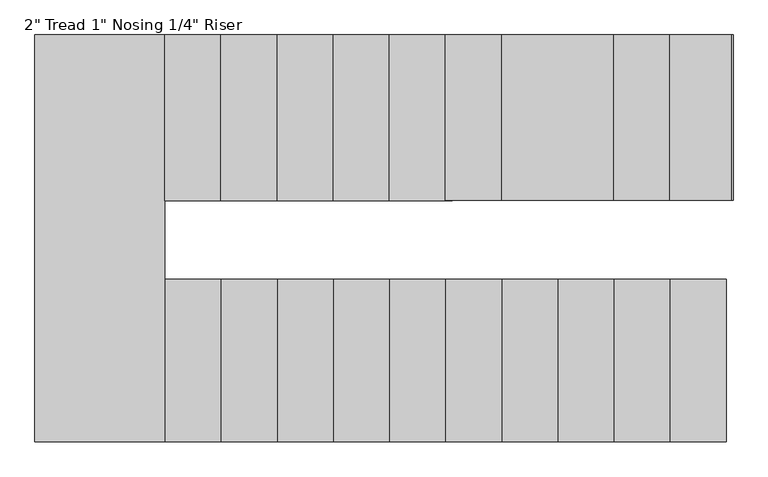
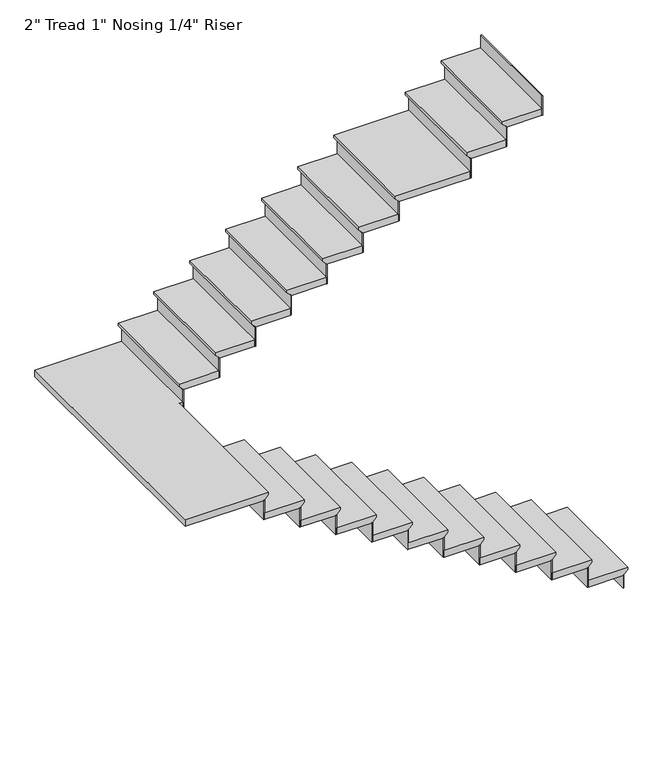
"""IFC4 building model written with IfcOpenShell, lengths in millimetres: stair flight geometry."""

from ifc_helpers import new_model, si_unit, origin, place, context, project, spatial, faceted_brep, source, transform, mapped, element, save


def stair_flight_03342cd4(model_context):
    return source(origin(), model_context, "Body", "Brep", [
        faceted_brep([(-3117.2664982, -7431.6600272, 9270.0928571), (-3117.2664982, -7431.6600272, 9289.1428571), (-3117.2664982, -8168.2600272, 9289.1428571), (-3117.2664982, -8168.2600272, 9270.0928571), (-3142.6664982, -7431.6600272, 9244.6928571), (-3142.6664982, -8168.2600272, 9244.6928571), (-3396.6664982, -7431.6600272, 9289.1428571), (-3396.6664982, -8168.2600272, 9289.1428571), (-3142.6664982, -8168.2600272, 9238.3428571), (-3396.6664982, -8168.2600272, 9238.3428571), (-3396.6664982, -7431.6600272, 9238.3428571), (-3142.6664982, -7431.6600272, 9238.3428571)], [[[0, 1, 2, 3]], [[4, 0, 3, 5]], [[2, 1, 6, 7]], [[8, 9, 10, 11]], [[2, 7, 9, 8, 5, 3]], [[8, 11, 4, 5]], [[6, 1, 0, 4, 11, 10]], [[7, 6, 10, 9]]]),
        faceted_brep([(-3142.6664982, -7431.6600272, 9238.3428571), (-3142.6664982, -7431.6600272, 9144.0), (-3149.0164982, -7431.6600272, 9144.0), (-3149.0164982, -7431.6600272, 9238.3428571), (-3142.6664982, -8168.2600272, 9238.3428571), (-3149.0164982, -8168.2600272, 9238.3428571), (-3149.0164982, -8168.2600272, 9144.0), (-3142.6664982, -8168.2600272, 9144.0)], [[[0, 1, 2, 3]], [[4, 5, 6, 7]], [[1, 0, 4, 7]], [[2, 1, 7, 6]], [[3, 2, 6, 5]], [[0, 3, 5, 4]]]),
        faceted_brep([(-3396.6664982, -7431.6600272, 9383.4857143), (-3396.6664982, -7431.6600272, 9238.3428571), (-3403.0164982, -7431.6600272, 9238.3428571), (-3403.0164982, -7431.6600272, 9383.4857143), (-3396.6664982, -8168.2600272, 9383.4857143), (-3403.0164982, -8168.2600272, 9383.4857143), (-3403.0164982, -8168.2600272, 9238.3428571), (-3396.6664982, -8168.2600272, 9238.3428571)], [[[0, 1, 2, 3]], [[4, 5, 6, 7]], [[1, 0, 4, 7]], [[2, 1, 7, 6]], [[3, 2, 6, 5]], [[0, 3, 5, 4]]]),
        faceted_brep([(-3371.2664982, -8168.2600272, 9434.2857143), (-3371.2664982, -7431.6600272, 9434.2857143), (-3650.6664982, -7431.6600272, 9434.2857143), (-3650.6664982, -8168.2600272, 9434.2857143), (-3396.6664982, -8168.2600272, 9383.4857143), (-3650.6664982, -8168.2600272, 9383.4857143), (-3650.6664982, -7431.6600272, 9383.4857143), (-3396.6664982, -7431.6600272, 9383.4857143), (-3396.6664982, -8168.2600272, 9389.8357143), (-3371.2664982, -8168.2600272, 9415.2357143), (-3396.6664982, -7431.6600272, 9389.8357143), (-3371.2664982, -7431.6600272, 9415.2357143)], [[[0, 1, 2, 3]], [[4, 5, 6, 7]], [[0, 3, 5, 4, 8, 9]], [[4, 7, 10, 8]], [[2, 1, 11, 10, 7, 6]], [[3, 2, 6, 5]], [[11, 1, 0, 9]], [[10, 11, 9, 8]]]),
        faceted_brep([(-3650.6664982, -7431.6600272, 9528.6285714), (-3650.6664982, -7431.6600272, 9383.4857143), (-3657.0164982, -7431.6600272, 9383.4857143), (-3657.0164982, -7431.6600272, 9528.6285714), (-3650.6664982, -8168.2600272, 9528.6285714), (-3657.0164982, -8168.2600272, 9528.6285714), (-3657.0164982, -8168.2600272, 9383.4857143), (-3650.6664982, -8168.2600272, 9383.4857143)], [[[0, 1, 2, 3]], [[4, 5, 6, 7]], [[1, 0, 4, 7]], [[2, 1, 7, 6]], [[3, 2, 6, 5]], [[0, 3, 5, 4]]]),
        faceted_brep([(-3625.2664982, -8168.2600272, 9579.4285714), (-3625.2664982, -7431.6600272, 9579.4285714), (-3904.6664982, -7431.6600272, 9579.4285714), (-3904.6664982, -8168.2600272, 9579.4285714), (-3650.6664982, -8168.2600272, 9528.6285714), (-3904.6664982, -8168.2600272, 9528.6285714), (-3904.6664982, -7431.6600272, 9528.6285714), (-3650.6664982, -7431.6600272, 9528.6285714), (-3650.6664982, -8168.2600272, 9534.9785714), (-3625.2664982, -8168.2600272, 9560.3785714), (-3650.6664982, -7431.6600272, 9534.9785714), (-3625.2664982, -7431.6600272, 9560.3785714)], [[[0, 1, 2, 3]], [[4, 5, 6, 7]], [[0, 3, 5, 4, 8, 9]], [[4, 7, 10, 8]], [[2, 1, 11, 10, 7, 6]], [[3, 2, 6, 5]], [[11, 1, 0, 9]], [[10, 11, 9, 8]]]),
        faceted_brep([(-3904.6664982, -7431.6600272, 9673.7714286), (-3904.6664982, -7431.6600272, 9528.6285714), (-3911.0164982, -7431.6600272, 9528.6285714), (-3911.0164982, -7431.6600272, 9673.7714286), (-3904.6664982, -8168.2600272, 9673.7714286), (-3911.0164982, -8168.2600272, 9673.7714286), (-3911.0164982, -8168.2600272, 9528.6285714), (-3904.6664982, -8168.2600272, 9528.6285714)], [[[0, 1, 2, 3]], [[4, 5, 6, 7]], [[1, 0, 4, 7]], [[2, 1, 7, 6]], [[3, 2, 6, 5]], [[0, 3, 5, 4]]]),
        faceted_brep([(-3879.2664982, -8168.2600272, 9724.5714286), (-3879.2664982, -7431.6600272, 9724.5714286), (-4158.6664982, -7431.6600272, 9724.5714286), (-4158.6664982, -8168.2600272, 9724.5714286), (-3904.6664982, -8168.2600272, 9673.7714286), (-4158.6664982, -8168.2600272, 9673.7714286), (-4158.6664982, -7431.6600272, 9673.7714286), (-3904.6664982, -7431.6600272, 9673.7714286), (-3904.6664982, -8168.2600272, 9680.1214286), (-3879.2664982, -8168.2600272, 9705.5214286), (-3904.6664982, -7431.6600272, 9680.1214286), (-3879.2664982, -7431.6600272, 9705.5214286)], [[[0, 1, 2, 3]], [[4, 5, 6, 7]], [[0, 3, 5, 4, 8, 9]], [[4, 7, 10, 8]], [[2, 1, 11, 10, 7, 6]], [[3, 2, 6, 5]], [[11, 1, 0, 9]], [[10, 11, 9, 8]]]),
        faceted_brep([(-4158.6664982, -7431.6600272, 9818.9142857), (-4158.6664982, -7431.6600272, 9673.7714286), (-4165.0164982, -7431.6600272, 9673.7714286), (-4165.0164982, -7431.6600272, 9818.9142857), (-4158.6664982, -8168.2600272, 9818.9142857), (-4165.0164982, -8168.2600272, 9818.9142857), (-4165.0164982, -8168.2600272, 9673.7714286), (-4158.6664982, -8168.2600272, 9673.7714286)], [[[0, 1, 2, 3]], [[4, 5, 6, 7]], [[1, 0, 4, 7]], [[2, 1, 7, 6]], [[3, 2, 6, 5]], [[0, 3, 5, 4]]]),
        faceted_brep([(-4133.2664982, -8168.2600272, 9869.7142857), (-4133.2664982, -7431.6600272, 9869.7142857), (-4412.6664982, -7431.6600272, 9869.7142857), (-4412.6664982, -8168.2600272, 9869.7142857), (-4158.6664982, -8168.2600272, 9818.9142857), (-4412.6664982, -8168.2600272, 9818.9142857), (-4412.6664982, -7431.6600272, 9818.9142857), (-4158.6664982, -7431.6600272, 9818.9142857), (-4158.6664982, -8168.2600272, 9825.2642857), (-4133.2664982, -8168.2600272, 9850.6642857), (-4158.6664982, -7431.6600272, 9825.2642857), (-4133.2664982, -7431.6600272, 9850.6642857)], [[[0, 1, 2, 3]], [[4, 5, 6, 7]], [[0, 3, 5, 4, 8, 9]], [[4, 7, 10, 8]], [[2, 1, 11, 10, 7, 6]], [[3, 2, 6, 5]], [[11, 1, 0, 9]], [[10, 11, 9, 8]]]),
        faceted_brep([(-4412.6664982, -7431.6600272, 9964.0571429), (-4412.6664982, -7431.6600272, 9818.9142857), (-4419.0164982, -7431.6600272, 9818.9142857), (-4419.0164982, -7431.6600272, 9964.0571429), (-4412.6664982, -8168.2600272, 9964.0571429), (-4419.0164982, -8168.2600272, 9964.0571429), (-4419.0164982, -8168.2600272, 9818.9142857), (-4412.6664982, -8168.2600272, 9818.9142857)], [[[0, 1, 2, 3]], [[4, 5, 6, 7]], [[1, 0, 4, 7]], [[2, 1, 7, 6]], [[3, 2, 6, 5]], [[0, 3, 5, 4]]]),
        faceted_brep([(-4387.2664982, -8168.2600272, 10014.8571429), (-4387.2664982, -7431.6600272, 10014.8571429), (-4666.6664982, -7431.6600272, 10014.8571429), (-4666.6664982, -8168.2600272, 10014.8571429), (-4412.6664982, -8168.2600272, 9964.0571429), (-4666.6664982, -8168.2600272, 9964.0571429), (-4666.6664982, -7431.6600272, 9964.0571429), (-4412.6664982, -7431.6600272, 9964.0571429), (-4412.6664982, -8168.2600272, 9970.4071429), (-4387.2664982, -8168.2600272, 9995.8071429), (-4412.6664982, -7431.6600272, 9970.4071429), (-4387.2664982, -7431.6600272, 9995.8071429)], [[[0, 1, 2, 3]], [[4, 5, 6, 7]], [[0, 3, 5, 4, 8, 9]], [[4, 7, 10, 8]], [[2, 1, 11, 10, 7, 6]], [[3, 2, 6, 5]], [[11, 1, 0, 9]], [[10, 11, 9, 8]]]),
        faceted_brep([(-4666.6664982, -7431.6600272, 10109.2), (-4666.6664982, -7431.6600272, 9964.0571429), (-4673.0164982, -7431.6600272, 9964.0571429), (-4673.0164982, -7431.6600272, 10109.2), (-4666.6664982, -8168.2600272, 10109.2), (-4673.0164982, -8168.2600272, 10109.2), (-4673.0164982, -8168.2600272, 9964.0571429), (-4666.6664982, -8168.2600272, 9964.0571429)], [[[0, 1, 2, 3]], [[4, 5, 6, 7]], [[1, 0, 4, 7]], [[2, 1, 7, 6]], [[3, 2, 6, 5]], [[0, 3, 5, 4]]]),
        faceted_brep([(-4641.2664982, -8168.2600272, 10160.0), (-4641.2664982, -7431.6600272, 10160.0), (-4920.6664982, -7431.6600272, 10160.0), (-4920.6664982, -8168.2600272, 10160.0), (-4666.6664982, -8168.2600272, 10109.2), (-4920.6664982, -8168.2600272, 10109.2), (-4920.6664982, -7431.6600272, 10109.2), (-4666.6664982, -7431.6600272, 10109.2), (-4666.6664982, -8168.2600272, 10115.55), (-4641.2664982, -8168.2600272, 10140.95), (-4666.6664982, -7431.6600272, 10115.55), (-4641.2664982, -7431.6600272, 10140.95)], [[[0, 1, 2, 3]], [[4, 5, 6, 7]], [[0, 3, 5, 4, 8, 9]], [[4, 7, 10, 8]], [[2, 1, 11, 10, 7, 6]], [[3, 2, 6, 5]], [[11, 1, 0, 9]], [[10, 11, 9, 8]]]),
        faceted_brep([(-4920.6664982, -7431.6600272, 10254.3428571), (-4920.6664982, -7431.6600272, 10109.2), (-4927.0164982, -7431.6600272, 10109.2), (-4927.0164982, -7431.6600272, 10254.3428571), (-4920.6664982, -8168.2600272, 10254.3428571), (-4927.0164982, -8168.2600272, 10254.3428571), (-4927.0164982, -8168.2600272, 10109.2), (-4920.6664982, -8168.2600272, 10109.2)], [[[0, 1, 2, 3]], [[4, 5, 6, 7]], [[1, 0, 4, 7]], [[2, 1, 7, 6]], [[3, 2, 6, 5]], [[0, 3, 5, 4]]]),
        faceted_brep([(-4895.2664982, -8168.2600272, 10305.1428571), (-4895.2664982, -7431.6600272, 10305.1428571), (-5174.6664982, -7431.6600272, 10305.1428571), (-5174.6664982, -8168.2600272, 10305.1428571), (-4920.6664982, -8168.2600272, 10254.3428571), (-5174.6664982, -8168.2600272, 10254.3428571), (-5174.6664982, -7431.6600272, 10254.3428571), (-4920.6664982, -7431.6600272, 10254.3428571), (-4920.6664982, -8168.2600272, 10260.6928571), (-4895.2664982, -8168.2600272, 10286.0928571), (-4920.6664982, -7431.6600272, 10260.6928571), (-4895.2664982, -7431.6600272, 10286.0928571)], [[[0, 1, 2, 3]], [[4, 5, 6, 7]], [[0, 3, 5, 4, 8, 9]], [[4, 7, 10, 8]], [[2, 1, 11, 10, 7, 6]], [[3, 2, 6, 5]], [[11, 1, 0, 9]], [[10, 11, 9, 8]]]),
        faceted_brep([(-5174.6664982, -7431.6600272, 10399.4857143), (-5174.6664982, -7431.6600272, 10254.3428571), (-5181.0164982, -7431.6600272, 10254.3428571), (-5181.0164982, -7431.6600272, 10399.4857143), (-5174.6664982, -8168.2600272, 10399.4857143), (-5181.0164982, -8168.2600272, 10399.4857143), (-5181.0164982, -8168.2600272, 10254.3428571), (-5174.6664982, -8168.2600272, 10254.3428571)], [[[0, 1, 2, 3]], [[4, 5, 6, 7]], [[1, 0, 4, 7]], [[2, 1, 7, 6]], [[3, 2, 6, 5]], [[0, 3, 5, 4]]]),
        faceted_brep([(-5149.2664982, -8168.2600272, 10450.2857143), (-5149.2664982, -7431.6600272, 10450.2857143), (-5428.6664982, -7431.6600272, 10450.2857143), (-5428.6664982, -8168.2600272, 10450.2857143), (-5174.6664982, -8168.2600272, 10399.4857143), (-5428.6664982, -8168.2600272, 10399.4857143), (-5428.6664982, -7431.6600272, 10399.4857143), (-5174.6664982, -7431.6600272, 10399.4857143), (-5174.6664982, -8168.2600272, 10405.8357143), (-5149.2664982, -8168.2600272, 10431.2357143), (-5174.6664982, -7431.6600272, 10405.8357143), (-5149.2664982, -7431.6600272, 10431.2357143)], [[[0, 1, 2, 3]], [[4, 5, 6, 7]], [[0, 3, 5, 4, 8, 9]], [[4, 7, 10, 8]], [[2, 1, 11, 10, 7, 6]], [[3, 2, 6, 5]], [[11, 1, 0, 9]], [[10, 11, 9, 8]]]),
        faceted_brep([(-5428.6664982, -7431.6600272, 10544.6285714), (-5428.6664982, -7431.6600272, 10399.4857143), (-5435.0164982, -7431.6600272, 10399.4857143), (-5435.0164982, -7431.6600272, 10544.6285714), (-5428.6664982, -8168.2600272, 10544.6285714), (-5435.0164982, -8168.2600272, 10544.6285714), (-5435.0164982, -8168.2600272, 10399.4857143), (-5428.6664982, -8168.2600272, 10399.4857143)], [[[0, 1, 2, 3]], [[4, 5, 6, 7]], [[1, 0, 4, 7]], [[2, 1, 7, 6]], [[3, 2, 6, 5]], [[0, 3, 5, 4]]]),
        faceted_brep([(-5403.2664982, -8168.2600272, 10595.4285714), (-5403.2664982, -7431.6600272, 10595.4285714), (-5682.6664982, -7431.6600272, 10595.4285714), (-5682.6664982, -8168.2600272, 10595.4285714), (-5428.6664982, -8168.2600272, 10544.6285714), (-5682.6664982, -8168.2600272, 10544.6285714), (-5682.6664982, -7431.6600272, 10544.6285714), (-5428.6664982, -7431.6600272, 10544.6285714), (-5428.6664982, -8168.2600272, 10550.9785714), (-5403.2664982, -8168.2600272, 10576.3785714), (-5428.6664982, -7431.6600272, 10550.9785714), (-5403.2664982, -7431.6600272, 10576.3785714)], [[[0, 1, 2, 3]], [[4, 5, 6, 7]], [[0, 3, 5, 4, 8, 9]], [[4, 7, 10, 8]], [[2, 1, 11, 10, 7, 6]], [[3, 2, 6, 5]], [[11, 1, 0, 9]], [[10, 11, 9, 8]]]),
        faceted_brep([(-5682.6664982, -7431.6600272, 10689.7714286), (-5682.6664982, -7431.6600272, 10544.6285714), (-5689.0164982, -7431.6600272, 10544.6285714), (-5689.0164982, -7431.6600272, 10689.7714286), (-5682.6664982, -8168.2600272, 10689.7714286), (-5689.0164982, -8168.2600272, 10689.7714286), (-5689.0164982, -8168.2600272, 10544.6285714), (-5682.6664982, -8168.2600272, 10544.6285714)], [[[0, 1, 2, 3]], [[4, 5, 6, 7]], [[1, 0, 4, 7]], [[2, 1, 7, 6]], [[3, 2, 6, 5]], [[0, 3, 5, 4]]]),
        faceted_brep([(-5631.8664982, -6326.7600272, 10740.5714286), (-6245.2108866, -6326.7600272, 10740.5714286), (-6245.2108866, -8168.2600272, 10740.5714286), (-5657.2664982, -8168.2600272, 10740.5714286), (-5657.2664982, -7076.0600272, 10740.5714286), (-5631.8664982, -7076.0600272, 10740.5714286), (-6245.2108866, -6326.7600272, 10689.7714286), (-5631.8664982, -6326.7600272, 10689.7714286), (-5631.8664982, -7076.0600272, 10689.7714286), (-5657.2664982, -7076.0600272, 10689.7714286), (-5657.2664982, -7431.6600272, 10689.7714286), (-5682.6664982, -7431.6600272, 10689.7714286), (-5682.6664982, -8168.2600272, 10689.7714286), (-6245.2108866, -8168.2600272, 10689.7714286), (-5682.6664982, -8168.2600272, 10696.1214286), (-5657.2664982, -8168.2600272, 10721.5214286), (-5682.6664982, -7431.6600272, 10696.1214286), (-5657.2664982, -7431.6600272, 10721.5214286)], [[[0, 1, 2, 3, 4, 5]], [[6, 7, 8, 9, 10, 11, 12, 13]], [[1, 0, 7, 6]], [[2, 1, 6, 13]], [[3, 2, 13, 12, 14, 15]], [[12, 11, 16, 14]], [[11, 10, 17, 16]], [[4, 3, 15, 17, 10, 9]], [[5, 4, 9, 8]], [[0, 5, 8, 7]], [[15, 14, 16, 17]]]),
        faceted_brep([(-5631.8664982, -7076.0600272, 10834.9142857), (-5631.8664982, -7076.0600272, 10689.7714286), (-5625.5164982, -7076.0600272, 10689.7714286), (-5625.5164982, -7076.0600272, 10834.9142857), (-5631.8664982, -6326.7600272, 10834.9142857), (-5625.5164982, -6326.7600272, 10834.9142857), (-5625.5164982, -6326.7600272, 10689.7714286), (-5631.8664982, -6326.7600272, 10689.7714286)], [[[0, 1, 2, 3]], [[4, 5, 6, 7]], [[1, 0, 4, 7]], [[2, 1, 7, 6]], [[3, 2, 6, 5]], [[0, 3, 5, 4]]]),
        faceted_brep([(-5657.2664982, -6326.7600272, 10885.7142857), (-5657.2664982, -7076.0600272, 10885.7142857), (-5377.8664982, -7076.0600272, 10885.7142857), (-5377.8664982, -6326.7600272, 10885.7142857), (-5631.8664982, -6326.7600272, 10834.9142857), (-5377.8664982, -6326.7600272, 10834.9142857), (-5377.8664982, -7076.0600272, 10834.9142857), (-5631.8664982, -7076.0600272, 10834.9142857), (-5631.8664982, -6326.7600272, 10841.2642857), (-5657.2664982, -6326.7600272, 10866.6642857), (-5631.8664982, -7076.0600272, 10841.2642857), (-5657.2664982, -7076.0600272, 10866.6642857)], [[[0, 1, 2, 3]], [[4, 5, 6, 7]], [[0, 3, 5, 4, 8, 9]], [[4, 7, 10, 8]], [[2, 1, 11, 10, 7, 6]], [[3, 2, 6, 5]], [[11, 1, 0, 9]], [[10, 11, 9, 8]]]),
        faceted_brep([(-5377.8664982, -7076.0600272, 10980.0571429), (-5377.8664982, -7076.0600272, 10834.9142857), (-5371.5164982, -7076.0600272, 10834.9142857), (-5371.5164982, -7076.0600272, 10980.0571429), (-5377.8664982, -6326.7600272, 10980.0571429), (-5371.5164982, -6326.7600272, 10980.0571429), (-5371.5164982, -6326.7600272, 10834.9142857), (-5377.8664982, -6326.7600272, 10834.9142857)], [[[0, 1, 2, 3]], [[4, 5, 6, 7]], [[1, 0, 4, 7]], [[2, 1, 7, 6]], [[3, 2, 6, 5]], [[0, 3, 5, 4]]]),
        faceted_brep([(-5403.2664982, -6326.7600272, 11030.8571429), (-5403.2664982, -7076.0600272, 11030.8571429), (-5123.8664982, -7076.0600272, 11030.8571429), (-5123.8664982, -6326.7600272, 11030.8571429), (-5377.8664982, -6326.7600272, 10980.0571429), (-5123.8664982, -6326.7600272, 10980.0571429), (-5123.8664982, -7076.0600272, 10980.0571429), (-5377.8664982, -7076.0600272, 10980.0571429), (-5377.8664982, -6326.7600272, 10986.4071429), (-5403.2664982, -6326.7600272, 11011.8071429), (-5377.8664982, -7076.0600272, 10986.4071429), (-5403.2664982, -7076.0600272, 11011.8071429)], [[[0, 1, 2, 3]], [[4, 5, 6, 7]], [[0, 3, 5, 4, 8, 9]], [[4, 7, 10, 8]], [[2, 1, 11, 10, 7, 6]], [[3, 2, 6, 5]], [[11, 1, 0, 9]], [[10, 11, 9, 8]]]),
        faceted_brep([(-5123.8664982, -7076.0600272, 11125.2), (-5123.8664982, -7076.0600272, 10980.0571429), (-5117.5164982, -7076.0600272, 10980.0571429), (-5117.5164982, -7076.0600272, 11125.2), (-5123.8664982, -6326.7600272, 11125.2), (-5117.5164982, -6326.7600272, 11125.2), (-5117.5164982, -6326.7600272, 10980.0571429), (-5123.8664982, -6326.7600272, 10980.0571429)], [[[0, 1, 2, 3]], [[4, 5, 6, 7]], [[1, 0, 4, 7]], [[2, 1, 7, 6]], [[3, 2, 6, 5]], [[0, 3, 5, 4]]]),
        faceted_brep([(-5149.2664982, -6326.7600272, 11176.0), (-5149.2664982, -7076.0600272, 11176.0), (-4869.8664982, -7076.0600272, 11176.0), (-4869.8664982, -6326.7600272, 11176.0), (-5123.8664982, -6326.7600272, 11125.2), (-4869.8664982, -6326.7600272, 11125.2), (-4869.8664982, -7076.0600272, 11125.2), (-5123.8664982, -7076.0600272, 11125.2), (-5123.8664982, -6326.7600272, 11131.55), (-5149.2664982, -6326.7600272, 11156.95), (-5123.8664982, -7076.0600272, 11131.55), (-5149.2664982, -7076.0600272, 11156.95)], [[[0, 1, 2, 3]], [[4, 5, 6, 7]], [[0, 3, 5, 4, 8, 9]], [[4, 7, 10, 8]], [[2, 1, 11, 10, 7, 6]], [[3, 2, 6, 5]], [[11, 1, 0, 9]], [[10, 11, 9, 8]]]),
        faceted_brep([(-4869.8664982, -7076.0600272, 11270.3428571), (-4869.8664982, -7076.0600272, 11125.2), (-4863.5164982, -7076.0600272, 11125.2), (-4863.5164982, -7076.0600272, 11270.3428571), (-4869.8664982, -6326.7600272, 11270.3428571), (-4863.5164982, -6326.7600272, 11270.3428571), (-4863.5164982, -6326.7600272, 11125.2), (-4869.8664982, -6326.7600272, 11125.2)], [[[0, 1, 2, 3]], [[4, 5, 6, 7]], [[1, 0, 4, 7]], [[2, 1, 7, 6]], [[3, 2, 6, 5]], [[0, 3, 5, 4]]]),
        faceted_brep([(-4895.2664982, -6326.7600272, 11321.1428571), (-4895.2664982, -7076.0600272, 11321.1428571), (-4615.8664982, -7076.0600272, 11321.1428571), (-4615.8664982, -6326.7600272, 11321.1428571), (-4869.8664982, -6326.7600272, 11270.3428571), (-4615.8664982, -6326.7600272, 11270.3428571), (-4615.8664982, -7076.0600272, 11270.3428571), (-4869.8664982, -7076.0600272, 11270.3428571), (-4869.8664982, -6326.7600272, 11276.6928571), (-4895.2664982, -6326.7600272, 11302.0928571), (-4869.8664982, -7076.0600272, 11276.6928571), (-4895.2664982, -7076.0600272, 11302.0928571)], [[[0, 1, 2, 3]], [[4, 5, 6, 7]], [[0, 3, 5, 4, 8, 9]], [[4, 7, 10, 8]], [[2, 1, 11, 10, 7, 6]], [[3, 2, 6, 5]], [[11, 1, 0, 9]], [[10, 11, 9, 8]]]),
        faceted_brep([(-4615.8664982, -7076.0600272, 11415.4857143), (-4615.8664982, -7076.0600272, 11270.3428571), (-4609.5164982, -7076.0600272, 11270.3428571), (-4609.5164982, -7076.0600272, 11415.4857143), (-4615.8664982, -6326.7600272, 11415.4857143), (-4609.5164982, -6326.7600272, 11415.4857143), (-4609.5164982, -6326.7600272, 11270.3428571), (-4615.8664982, -6326.7600272, 11270.3428571)], [[[0, 1, 2, 3]], [[4, 5, 6, 7]], [[1, 0, 4, 7]], [[2, 1, 7, 6]], [[3, 2, 6, 5]], [[0, 3, 5, 4]]]),
        faceted_brep([(-4641.2664982, -6326.7600272, 11466.2857143), (-4641.2664982, -7076.0600272, 11466.2857143), (-4361.8664982, -7076.0600272, 11466.2857143), (-4361.8664982, -6326.7600272, 11466.2857143), (-4615.8664982, -6326.7600272, 11415.4857143), (-4361.8664982, -6326.7600272, 11415.4857143), (-4361.8664982, -7076.0600272, 11415.4857143), (-4615.8664982, -7076.0600272, 11415.4857143), (-4615.8664982, -6326.7600272, 11421.8357143), (-4641.2664982, -6326.7600272, 11447.2357143), (-4615.8664982, -7076.0600272, 11421.8357143), (-4641.2664982, -7076.0600272, 11447.2357143)], [[[0, 1, 2, 3]], [[4, 5, 6, 7]], [[0, 3, 5, 4, 8, 9]], [[4, 7, 10, 8]], [[2, 1, 11, 10, 7, 6]], [[3, 2, 6, 5]], [[11, 1, 0, 9]], [[10, 11, 9, 8]]]),
        faceted_brep([(-4361.8664982, -7076.0600272, 11560.6285714), (-4361.8664982, -7076.0600272, 11415.4857143), (-4355.5164982, -7076.0600272, 11415.4857143), (-4355.5164982, -7076.0600272, 11560.6285714), (-4361.8664982, -6326.7600272, 11560.6285714), (-4355.5164982, -6326.7600272, 11560.6285714), (-4355.5164982, -6326.7600272, 11415.4857143), (-4361.8664982, -6326.7600272, 11415.4857143)], [[[0, 1, 2, 3]], [[4, 5, 6, 7]], [[1, 0, 4, 7]], [[2, 1, 7, 6]], [[3, 2, 6, 5]], [[0, 3, 5, 4]]]),
        faceted_brep([(-4387.2664982, -6326.7600272, 11611.4285714), (-4387.2664982, -7076.0600272, 11611.4285714), (-4107.8664982, -7076.0600272, 11611.4285714), (-4107.8664982, -6326.7600272, 11611.4285714), (-4361.8664982, -6326.7600272, 11560.6285714), (-4107.8664982, -6326.7600272, 11560.6285714), (-4107.8664982, -7076.0600272, 11560.6285714), (-4361.8664982, -7076.0600272, 11560.6285714), (-4361.8664982, -6326.7600272, 11566.9785714), (-4387.2664982, -6326.7600272, 11592.3785714), (-4361.8664982, -7076.0600272, 11566.9785714), (-4387.2664982, -7076.0600272, 11592.3785714)], [[[0, 1, 2, 3]], [[4, 5, 6, 7]], [[0, 3, 5, 4, 8, 9]], [[4, 7, 10, 8]], [[2, 1, 11, 10, 7, 6]], [[3, 2, 6, 5]], [[11, 1, 0, 9]], [[10, 11, 9, 8]]]),
        faceted_brep([(-4107.8664982, -7076.0600272, 11705.7714286), (-4107.8664982, -7076.0600272, 11560.6285714), (-4101.5164982, -7076.0600272, 11560.6285714), (-4101.5164982, -7076.0600272, 11705.7714286), (-4107.8664982, -6326.7600272, 11705.7714286), (-4101.5164982, -6326.7600272, 11705.7714286), (-4101.5164982, -6326.7600272, 11560.6285714), (-4107.8664982, -6326.7600272, 11560.6285714)], [[[0, 1, 2, 3]], [[4, 5, 6, 7]], [[1, 0, 4, 7]], [[2, 1, 7, 6]], [[3, 2, 6, 5]], [[0, 3, 5, 4]]]),
        faceted_brep([(-4133.2664982, -6326.7600272, 11756.5714286), (-4133.2664982, -7076.0600272, 11756.5714286), (-3599.8664982, -7076.0600272, 11756.5714286), (-3599.8664982, -6326.7600272, 11756.5714286), (-4107.8664982, -6326.7600272, 11705.7714286), (-3599.8664982, -6326.7600272, 11705.7714286), (-3599.8664982, -7076.0600272, 11705.7714286), (-4107.8664982, -7076.0600272, 11705.7714286), (-4107.8664982, -6326.7600272, 11712.1214286), (-4133.2664982, -6326.7600272, 11737.5214286), (-4107.8664982, -7076.0600272, 11712.1214286), (-4133.2664982, -7076.0600272, 11737.5214286)], [[[0, 1, 2, 3]], [[4, 5, 6, 7]], [[0, 3, 5, 4, 8, 9]], [[4, 7, 10, 8]], [[2, 1, 11, 10, 7, 6]], [[3, 2, 6, 5]], [[11, 1, 0, 9]], [[10, 11, 9, 8]]]),
        faceted_brep([(-3599.8664982, -7076.0600272, 11850.9142857), (-3599.8664982, -7076.0600272, 11705.7714286), (-3593.5164982, -7076.0600272, 11705.7714286), (-3593.5164982, -7076.0600272, 11850.9142857), (-3599.8664982, -6326.7600272, 11850.9142857), (-3593.5164982, -6326.7600272, 11850.9142857), (-3593.5164982, -6326.7600272, 11705.7714286), (-3599.8664982, -6326.7600272, 11705.7714286)], [[[0, 1, 2, 3]], [[4, 5, 6, 7]], [[1, 0, 4, 7]], [[2, 1, 7, 6]], [[3, 2, 6, 5]], [[0, 3, 5, 4]]]),
        faceted_brep([(-3625.2664982, -6326.7600272, 11901.7142857), (-3625.2664982, -7076.0600272, 11901.7142857), (-3345.8664982, -7076.0600272, 11901.7142857), (-3345.8664982, -6326.7600272, 11901.7142857), (-3599.8664982, -6326.7600272, 11850.9142857), (-3345.8664982, -6326.7600272, 11850.9142857), (-3345.8664982, -7076.0600272, 11850.9142857), (-3599.8664982, -7076.0600272, 11850.9142857), (-3599.8664982, -6326.7600272, 11857.2642857), (-3625.2664982, -6326.7600272, 11882.6642857), (-3599.8664982, -7076.0600272, 11857.2642857), (-3625.2664982, -7076.0600272, 11882.6642857)], [[[0, 1, 2, 3]], [[4, 5, 6, 7]], [[0, 3, 5, 4, 8, 9]], [[4, 7, 10, 8]], [[2, 1, 11, 10, 7, 6]], [[3, 2, 6, 5]], [[11, 1, 0, 9]], [[10, 11, 9, 8]]]),
        faceted_brep([(-3345.8664982, -7076.0600272, 11996.0571429), (-3345.8664982, -7076.0600272, 11850.9142857), (-3339.5164982, -7076.0600272, 11850.9142857), (-3339.5164982, -7076.0600272, 11996.0571429), (-3345.8664982, -6326.7600272, 11996.0571429), (-3339.5164982, -6326.7600272, 11996.0571429), (-3339.5164982, -6326.7600272, 11850.9142857), (-3345.8664982, -6326.7600272, 11850.9142857)], [[[0, 1, 2, 3]], [[4, 5, 6, 7]], [[1, 0, 4, 7]], [[2, 1, 7, 6]], [[3, 2, 6, 5]], [[0, 3, 5, 4]]]),
        faceted_brep([(-3091.8664982, -7076.0600272, 12141.2), (-3091.8664982, -7076.0600272, 11996.0571429), (-3085.5164982, -7076.0600272, 11996.0571429), (-3085.5164982, -7076.0600272, 12141.2), (-3091.8664982, -6326.7600272, 12141.2), (-3085.5164982, -6326.7600272, 12141.2), (-3085.5164982, -6326.7600272, 11996.0571429), (-3091.8664982, -6326.7600272, 11996.0571429)], [[[0, 1, 2, 3]], [[4, 5, 6, 7]], [[1, 0, 4, 7]], [[2, 1, 7, 6]], [[3, 2, 6, 5]], [[0, 3, 5, 4]]]),
        faceted_brep([(-3371.2664982, -6326.7600272, 12046.8571429), (-3371.2664982, -7076.0600272, 12046.8571429), (-3091.8664982, -7076.0600272, 12046.8571429), (-3091.8664982, -6326.7600272, 12046.8571429), (-3345.8664982, -6326.7600272, 11996.0571429), (-3091.8664982, -6326.7600272, 11996.0571429), (-3091.8664982, -7076.0600272, 11996.0571429), (-3345.8664982, -7076.0600272, 11996.0571429), (-3345.8664982, -6326.7600272, 12002.4071429), (-3371.2664982, -6326.7600272, 12027.8071429), (-3345.8664982, -7076.0600272, 12002.4071429), (-3371.2664982, -7076.0600272, 12027.8071429)], [[[0, 1, 2, 3]], [[4, 5, 6, 7]], [[0, 3, 5, 4, 8, 9]], [[4, 7, 10, 8]], [[2, 1, 11, 10, 7, 6]], [[3, 2, 6, 5]], [[11, 1, 0, 9]], [[10, 11, 9, 8]]]),
    ])


if __name__ == "__main__":
    model = new_model("IFC4")
    model_context = context("Model", 3, world=origin())
    ifc_project = project(units=[si_unit("LENGTHUNIT", "METRE", prefix="MILLI")], contexts=[model_context])
    site = spatial("IfcSite", under=ifc_project)
    building = spatial("IfcBuilding", under=site)
    placement = place(None, origin())
    stair_flight_shape = stair_flight_03342cd4(model_context)
    element("IfcStairFlight", 1, ObjectType="2\" Tread 1\" Nosing 1/4\" Riser", at=placement, inside=building, context=model_context, shape_type="MappedRepresentation", body=[
        mapped(stair_flight_shape, transform((0.0, 0.0, 0.0), x_axis=(1.0, 0.0, 0.0), y_axis=(0.0, 1.0, 0.0), z_axis=(0.0, 0.0, 1.0))),
    ])
    save(model, "model.ifc")
